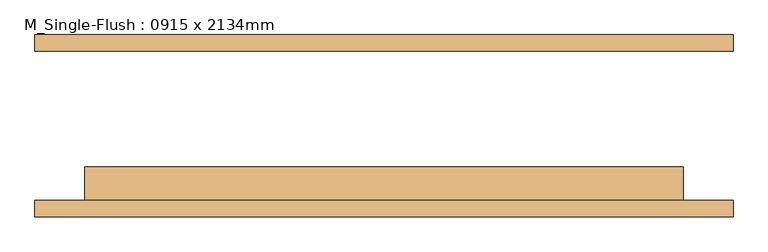
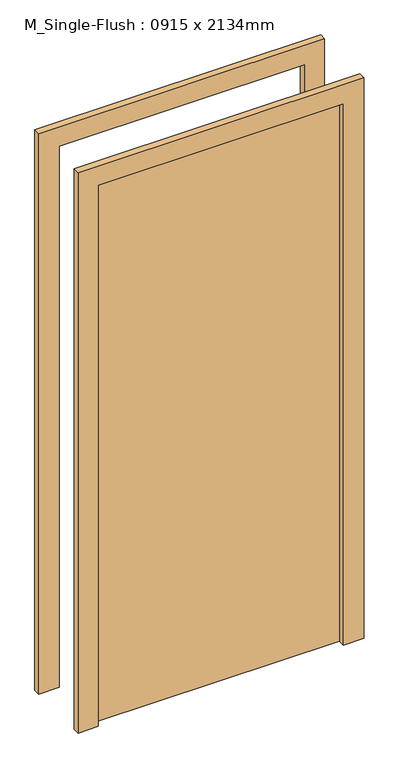
"""IFC4 building model written with IfcOpenShell, lengths in millimetres: door geometry, M_Single-Flush : 0915 x 2134mm."""

from ifc_helpers import new_model, si_unit, frame, origin, origin_with_axes, place, context, project, spatial, polyline, outline, extrude, source, transform, mapped, element, save


def m_single_flush_0915_x_2134mm_43602619(model_context):
    return source(origin(), model_context, "Body", "SweptSolid", [
        extrude(outline(polyline([(2210.0, -533.5), (0.0, -533.5), (0.0, -457.5), (2134.0, -457.5), (2134.0, 457.5), (0.0, 457.5), (0.0, 533.5), (2210.0, 533.5), (2210.0, -533.5)])), frame((0.0, -139.3, 0.0), z_axis=(0.0, 1.0, 0.0), x_axis=(0.0, 0.0, 1.0)), (0.0, 0.0, 1.0), 25.0),
        extrude(outline(polyline([(2210.0, 533.5), (2210.0, -533.5), (0.0, -533.5), (0.0, -457.5), (2134.0, -457.5), (2134.0, 457.5), (0.0, 457.5), (0.0, 533.5), (2210.0, 533.5)])), frame((0.0, 114.3, 0.0), z_axis=(0.0, 1.0, 0.0), x_axis=(0.0, 0.0, 1.0)), (0.0, 0.0, 1.0), 25.0),
        extrude(outline(polyline([(457.5, -63.3), (457.5, -114.3), (-457.5, -114.3), (-457.5, -63.3), (457.5, -63.3)])), origin_with_axes(), (0.0, 0.0, 1.0), 2134.0),
    ])


if __name__ == "__main__":
    model = new_model("IFC4")
    model_context = context("Model", 3, world=origin())
    ifc_project = project(units=[si_unit("LENGTHUNIT", "METRE", prefix="MILLI")], contexts=[model_context])
    site = spatial("IfcSite", under=ifc_project)
    building = spatial("IfcBuilding", under=site)
    placement = place(None, origin())
    m_single_flush_0915_x_2134mm_shape = m_single_flush_0915_x_2134mm_43602619(model_context)
    element("IfcDoor", 1, ObjectType="M_Single-Flush : 0915 x 2134mm", at=placement, inside=building, context=model_context, shape_type="MappedRepresentation", body=[
        mapped(m_single_flush_0915_x_2134mm_shape, transform((0.0, 0.0, 0.0), x_axis=(1.0, 0.0, 0.0), y_axis=(0.0, 1.0, 0.0), z_axis=(0.0, 0.0, 1.0))),
    ])
    save(model, "model.ifc")

# Revit data of these elements
# Type "M_Single-Flush : 0915 x 2134mm"
#   Type Mark = "20"
#   Construction Type Id = "MDOOR"
#   Analytic Construction = "Metal"
#   Thickness = 0.167323 ft
#   Thermal Resistance (R) = 0.270117 (m²·K)/W
#   Heat Transfer Coefficient (U) = 3.7021 W/(m²·K)
#   Height = 7.001312 ft
#   Trim Projection Ext = 0.082021 ft
#   Trim Projection Int = 0.082021 ft
#   Trim Width = 0.249344 ft
#   Width = 3.001969 ft
#   Define Thermal Properties by = 1
#   Define Thermal Properties by = 1
#   Door Material = Door - Panel
#   Frame Material = Door - Frame
#   Visual Light Transmittance = 0
#   Solar Heat Gain Coefficient = 0
#   Function = (empty or 0)
#   Wall Closure = (empty or 0)
# Element 1 (IfcDoor, "M_Single-Flush : 0915 x 2134mm")
#   Materials on its faces: "Door - Frame", "Door - Panel"
# Materials
#   "Door - Panel": class "Wood", colour RGB 210 159 95, transparency 0, Cost = 0
#   "Door - Frame": colour RGB 118 70 51, transparency 0, Cost = 0
